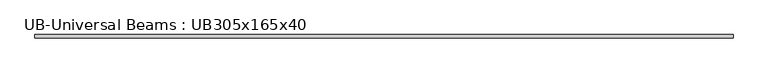
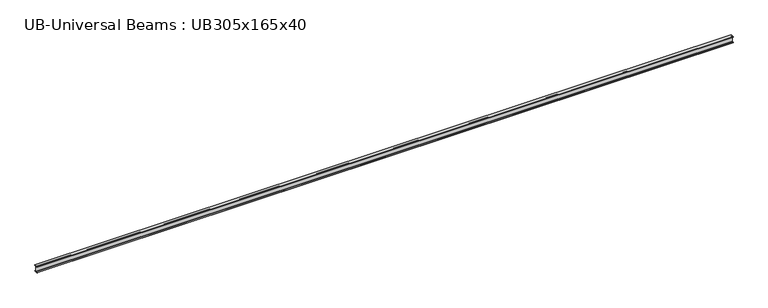
"""IFC4 building model written with IfcOpenShell, lengths in millimetres: beam geometry, UB-Universal Beams : UB305x165x40."""

from ifc_helpers import new_model, si_unit, point, frame, frame_2d, origin, place, context, project, spatial, polyline, circle_curve, trimmed, segment, composite_curve, outline, extrude, source, transform, mapped, element, save


def ub_universal_beams_ub305x165x40_e9518ab5(model_context):
    return source(origin(), model_context, "Body", "SweptSolid", [
        extrude(outline(composite_curve([segment(polyline([(82.5, -141.5), (82.5, -151.7), (-82.5, -151.7), (-82.5, -141.5), (-11.9, -141.5)]), True, "CONTINUOUS"), segment(trimmed(circle_curve(frame_2d((-11.9, -132.6)), 8.9), [point((-11.9, -141.5))], [point((-3.0, -132.6))], True, "CARTESIAN"), True, "CONTINUOUS"), segment(polyline([(-3.0, -132.6), (-3.0, 132.6)]), True, "CONTINUOUS"), segment(trimmed(circle_curve(frame_2d((-11.9, 132.6)), 8.9), [point((-3.0, 132.6))], [point((-11.9, 141.5))], True, "CARTESIAN"), True, "CONTINUOUS"), segment(polyline([(-11.9, 141.5), (-82.5, 141.5), (-82.5, 151.7), (82.5, 151.7), (82.5, 141.5), (11.9, 141.5)]), True, "CONTINUOUS"), segment(trimmed(circle_curve(frame_2d((11.9, 132.6)), 8.9), [point((11.9, 141.5))], [point((3.0, 132.6))], True, "CARTESIAN"), True, "CONTINUOUS"), segment(polyline([(3.0, 132.6), (3.0, -132.6)]), True, "CONTINUOUS"), segment(trimmed(circle_curve(frame_2d((11.9, -132.6)), 8.9), [point((3.0, -132.6))], [point((11.9, -141.5))], True, "CARTESIAN"), True, "CONTINUOUS"), segment(polyline([(11.9, -141.5), (82.5, -141.5)]), True, "CONTINUOUS")], self_intersect=False)), frame((-18370.5, 0.0, 0.0), z_axis=(1.0, 0.0, 0.0), x_axis=(0.0, 1.0, 0.0)), (0.0, 0.0, 1.0), 34323.9),
    ])


if __name__ == "__main__":
    model = new_model("IFC4")
    model_context = context("Model", 3, world=origin())
    ifc_project = project(units=[si_unit("LENGTHUNIT", "METRE", prefix="MILLI")], contexts=[model_context])
    site = spatial("IfcSite", under=ifc_project)
    building = spatial("IfcBuilding", under=site)
    placement = place(None, origin())
    ub_universal_beams_ub305x165x40_shape = ub_universal_beams_ub305x165x40_e9518ab5(model_context)
    element("IfcBeam", 1, ObjectType="UB-Universal Beams : UB305x165x40", at=placement, inside=building, context=model_context, shape_type="MappedRepresentation", body=[
        mapped(ub_universal_beams_ub305x165x40_shape, transform((0.0, 0.0, 0.0), x_axis=(1.0, 0.0, 0.0), y_axis=(0.0, 1.0, 0.0), z_axis=(0.0, 0.0, 1.0))),
    ])
    save(model, "model.ifc")

# Revit data of these elements
# Type "UB-Universal Beams : UB305x165x40"
#   Section Name Key = "UB305X165X40"
#   Width = 16.5 cm
#   Web Thickness = 0.6 cm
#   Web Fillet = 0.89 cm
#   Warping Constant = 164000.0 cm⁶
#   Torsional Moment of Inertia = 14.70 cm⁴
#   Section Area = 51.3 cm²
#   Plastic Modulus weak axis = 142.0 cm³
#   Plastic Modulus strong axis = 623.0 cm³
#   Nominal Weight = 40.2999 kgf/m
#   Moment of Inertia weak axis = 764.00 cm⁴
#   Moment of Inertia strong axis = 8503.00 cm⁴
#   Height = 30.34 cm
#   Flange Thickness = 1.02 cm
#   Elastic Modulus weak axis = 92.6 cm³
#   Elastic Modulus strong axis = 560.0 cm³
#   Centroid Vertical = 15.17 cm
#   Centroid Horizontal = 8.25 cm
#   Bolt Spacing = 9.0 cm
#   Length [instance default] = 1500 mm
#   Structural Material [instance default] = Metal - Steel 43-275
#   Type Comments = ""
#   Assembly Code = ""
# Element 1 (IfcBeam, "UB-Universal Beams : UB305x165x40")
#   Materials on its faces: "Metal - Steel 43-275"
# Materials
#   "Metal - Steel 43-275": class "Metal", colour RGB 247 247 247, transparency 0, Cost = 0
